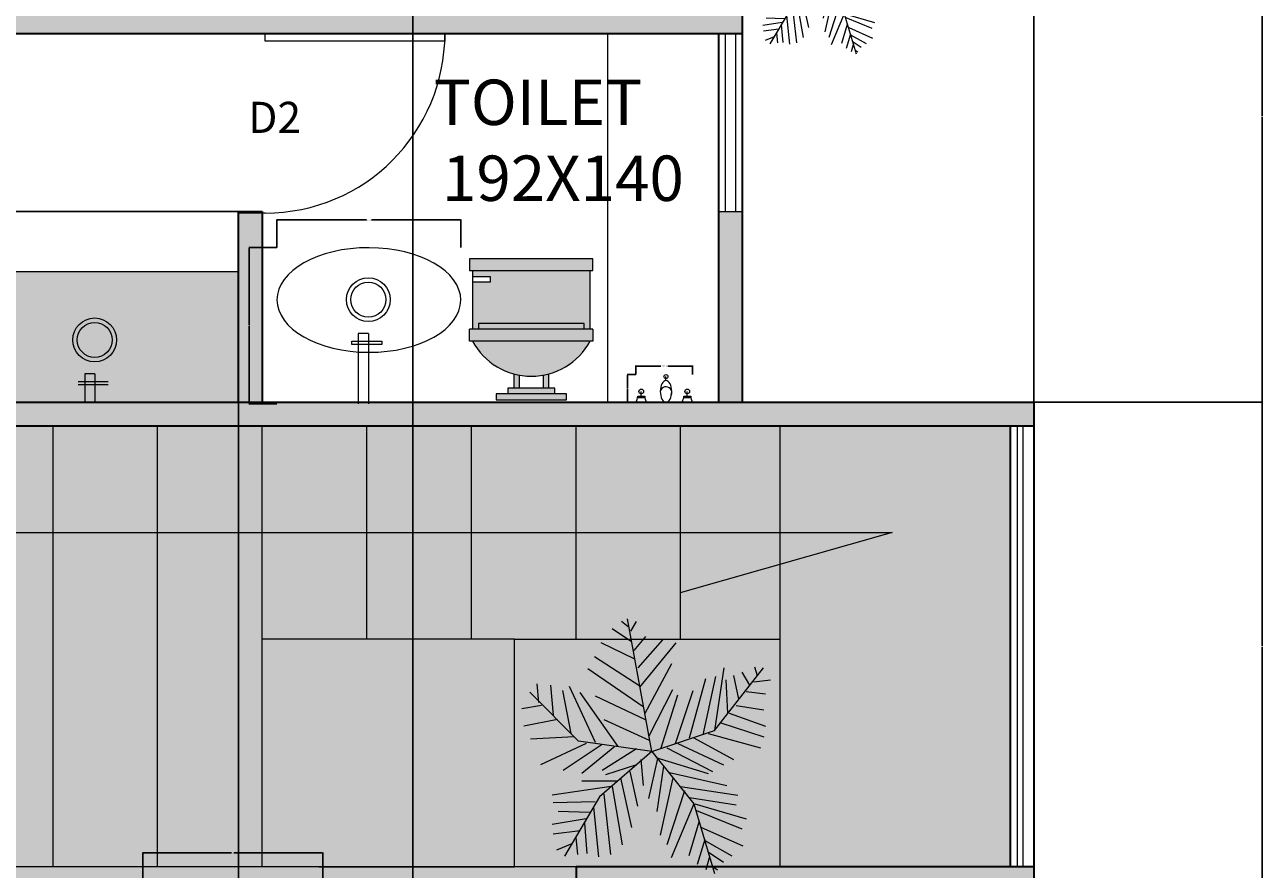
# Model space of a CAD drawing. Units: inches. Extents: x 192 to 1361, y -1362 to 367.
# Tile 13 of 23: x 891 to 1361, y -775 to -454. Entities that reach past the tile are written whole.
import ezdxf

# ---------------------------------------------------------------- set-up
doc = ezdxf.new("R2010")
doc.units = ezdxf.units.IN
doc.header["$MEASUREMENT"] = 0
for name, color, linetype, lineweight in [('A-ANNO-DIMS', 2, 'Continuous', 18), ('A-ANNO-SYMB', 7, 'Continuous', 18), ('A-AREA-IDEN', 7, 'Continuous', 18), ('A-DOOR', 4, 'Continuous', 18), ('A-FLOR-CASE', 32, 'Continuous', 18), ('A-FLOR-FIXT', 8, 'Continuous', 18), ('A-FLOR-STRS', 7, 'Continuous', 18), ('A-WALL-PATT', 250, 'Continuous', 13), ('lawn', 96, 'Continuous', 13), ('text', 7, 'Continuous', 18), ('walls', 7, 'Continuous', 35), ('windows', 4, 'Continuous', 18)]:
    doc.layers.add(name, color=color, linetype=linetype, lineweight=lineweight)
for name, color, linetype, lineweight, true_color in [('A-FLOR-CASE-PATT', 9, 'Continuous', 13, 0xc7c8ca), ('A-FLOR-FIXT-PATT', 251, 'Continuous', 13, 0x636466), ('A-FLOR-STRS-PATT', 252, 'Continuous', 13, 0x939598)]:
    doc.layers.add(name, color=color, linetype=linetype, lineweight=lineweight, true_color=true_color)
doc.styles.get("Standard").update_dxf_attribs({"font": 'arial.ttf'})
doc.dimstyles.get("Standard").update_dxf_attribs({"dimtxt": 0.18, "dimasz": 0.18, "dimexe": 0.18, "dimexo": 0.0625, "dimgap": 0.09, "dimtad": 0, "dimtih": 1, "dimtoh": 1, "dimzin": 0, "dimdsep": 46, "dimlunit": 3, "dimtxsty": 'Standard', "dimcen": 0.09, "dimadec": 0, "dimazin": 0, "dimtfac": 1, "dimtofl": 0, "dimtmove": 0, "dimatfit": 3, "dimfxl": 1, "dimtolj": 1, "dimtzin": 0, "dimarcsym": 0})

# ---------------------------------------------------------------- blocks, each defined once
blk = doc.blocks.new('*U2')
for p, q in [((0, 0), (0, -6)), ((40, 0), (40, -6))]:
    blk.add_line(p, q)
blk.add_lwpolyline([(0, 0), (0, 40), (1.75, 40), (1.75, 0)], close=True)
blk.add_arc((0, 0), 40, 0, 90)
blk = doc.blocks.new('*U4')
for p, q in [((-10.186, 53.64), (-13.084, 55.962)), ((0, 0), (-10.5, 57)), ((-9.099, 51.782), (-6.563, 55.962)), ((-8.737, 47.138), (-17.069, 52.711)), ((-7.65, 43.423), (-2.578, 49.46)), ((-5.839, 35.992), (4.667, 48.067)), ((-7.288, 39.707), (-21.778, 46.673)), ((-5.114, 27.632), (10.463, 46.673)), ((-5.114, 28.097), (-24.676, 40.636)), ((-2.941, 16.486), (8.652, 37.85)), ((-3.665, 19.273), (-27.574, 35.527)), ((22.055, 7.198), (27.489, 32.277)), ((27, 9), (48, 36)), ((27.127, 9.056), (31.112, 35.992)), ((35.096, 32.741), (37.27, 22.524)), ((38.719, 34.134), (41.979, 28.561)), ((44.153, 36.456), (45.239, 32.741)), ((-48.585, 21.131), (-49.309, 29.026)), ((-43.513, 28.561), (-42.427, 15.558)), ((-35.544, 28.097), (-24.314, 3.947)), ((-1.129, 6.734), (9.014, 26.704)), ((16.259, 5.805), (23.142, 31.348)), ((31.836, 30.883), (32.561, 16.486)), ((43.791, 29.954), (51.036, 30.883)), ((-31.5, 4.5), (-52.5, 25.5)), ((-38.442, 26.239), (-34.819, 7.663)), ((-14.533, 2.09), (-30.834, 25.31)), ((-24.314, 23.917), (-2.941, 13.7)), ((3.942, 1.625), (11.187, 24.381)), ((10.101, 3.483), (17.708, 26.239)), ((40.53, 25.775), (48.862, 24.846)), ((-47.498, 19.737), (-55.83, 18.344)), ((33.285, 16.486), (48.862, 10.913)), ((36.183, 19.737), (48.137, 17.88)), ((-40.615, 13.7), (-55.105, 10.913)), ((-20.691, 13.7), (-1.129, 4.876)), ((29.662, 12.307), (48.137, 6.269)), ((-33.37, 6.269), (-52.207, 5.34)), ((0, 0), (27, 9)), ((18.07, 5.805), (35.096, -3.483)), ((24.229, 7.663), (46.688, 1.625)), ((-28.299, 3.483), (-47.86, -5.805)), ((-21.416, 3.018), (-38.079, -8.128)), ((0, 0), (-31.5, 4.5)), ((-15.982, 2.09), (-30.11, -9.521)), ((0, 0), (-22.5, -19.5)), ((-6.563, 1.161), (-21.416, -8.128)), ((0, 0), (18, -22.5)), ((6.478, 1.625), (26.04, -8.592)), ((11.187, 3.483), (30.749, -5.805)), ((-4.752, -3.483), (-3.665, -14.629)), ((2.493, -3.019), (-1.491, -20.202)), ((1.769, -2.555), (24.229, -9.521)), ((-6.563, -5.805), (-19.967, -9.985)), ((-9.461, -8.592), (-6.201, -23.453)), ((5.029, -6.27), (2.131, -25.775)), ((7.565, -9.056), (32.198, -14.629)), ((-17.431, -15.094), (-42.789, -18.809)), ((-15.257, -12.772), (-30.11, -12.772)), ((-17.069, -15.094), (-12.721, -40.172)), ((-13.446, -11.378), (-8.737, -32.741)), ((9.014, -11.378), (3.58, -35.992)), ((12.274, -15.094), (36.907, -18.809)), ((-22.5, -19.5), (-37.5, -45)), ((-20.691, -18.345), (-17.793, -44.352)), ((14.085, -16.951), (6.478, -40.172)), ((16.259, -19.738), (36.183, -22.989)), ((-24.314, -21.596), (-42.427, -22.06)), ((-26.849, -26.24), (-40.253, -25.775)), ((-25.038, -23.918), (-22.865, -45.281)), ((18.07, -22.524), (8.289, -45.745)), ((18, -22.5), (27, -52.5)), ((18.433, -22.524), (40.53, -29.026)), ((19.157, -25.311), (38.719, -33.206)), ((-28.299, -29.026), (-42.789, -31.348)), ((-29.023, -30.884), (-27.936, -43.887)), ((20.244, -30.419), (15.897, -44.816)), ((-30.834, -34.135), (-42.427, -35.528)), ((-32.646, -36.921), (-31.921, -44.352)), ((21.331, -32.741), (39.081, -40.636)), ((-34.457, -39.708), (-40.978, -42.494)), ((22.78, -37.85), (19.519, -48.532)), ((22.78, -38.314), (34.372, -44.816)), ((24.591, -45.745), (23.142, -50.854)), ((24.591, -43.423), (30.749, -47.603)), ((26.764, -49.925), (28.213, -50.854))]:
    blk.add_line(p, q)
blk = doc.blocks.new('*U18')
for p, q in [((-10, 22), (-10, 12)), ((10, 12), (10, 22)), ((-10, 21), (-7, 21)), ((-7, 20), (-10, 20)), ((-7, 21), (-7, 20)), ((9, 13), (-9, 13)), ((-9, 13), (-9, 12)), ((9, 12), (9, 13)), ((10.5, 12), (-10.5, 12)), ((-10.5, 10), (-10.5, 12)), ((10.5, 12), (10.5, 10)), ((10.5, 10), (-10.5, 10)), ((-3, 4.4065), (-3, 2)), ((3, 2), (3, 4.4065)), ((-2, 2), (-2, 4.1658)), ((2, 4.1658), (2, 2)), ((4, 2), (-4, 2)), ((-4, 2), (-4, 1)), ((4, 1), (4, 2))]:
    blk.add_line(p, q)
for points in [[(10.5, 22), (10.5, 24), (-10.5, 24), (-10.5, 22)], [(6, 0), (6, 1), (-6, 1), (-6, 0)]]:
    blk.add_lwpolyline(points, close=True)
blk.add_arc((0, 15.3333), 11.3333, 208.0725, 331.9275)
blk = doc.blocks.new('BASIN-OVAL-WITH-TAP')
for p, q in [((-0.13, -12.72), (-4, -12.74)), ((-4, -12.74), (-4, -39.43)), ((-0.13, -12.72), (-0.13, -39.43)), ((-6.48, -15.66), (4.91, -15.61)), ((-6.47, -16.92), (-6.48, -15.66)), ((4.94, -16.86), (-6.47, -16.92))]:
    blk.add_line(p, q)
for radius in [8.31, 6.64]:
    blk.add_circle((-0.19, 0.14), radius)
at = {"extrusion": (0, 0, -1)}
blk.add_ellipse((0, 0), major_axis=(-34.9, 0.1), ratio=0.56899, dxfattribs=at)
blk = doc.blocks.new('BATH-MIXER-TWIN-HANDLE')
for p, q in [((0, 4.11), (0, 5.63)), ((-10.73, -2.32), (-8.02, -2.36)), ((-10.7, -1.84), (-8.05, -1.84)), ((-9.38, -1.84), (-9.38, -0.03)), ((6.73, -2.31), (9.44, -2.32)), ((6.76, -1.84), (9.41, -1.84)), ((8.08, -1.84), (8.08, -0.03))]:
    blk.add_line(p, q)
for centre, radius in [((0, 5.63), 0.761), ((-9.38, -0.03), 0.904), ((8.08, -0.03), 0.904)]:
    blk.add_circle(centre, radius)
for centre, radius, start, end in [((0, -0.5), 2.23, 336.3452, 166.942), ((-14.82, -1.84), 4.11, 326.5495, 0), ((-3.94, -1.84), 4.11, 180, 213.4505), ((2.65, -1.84), 4.11, 326.5495, 0), ((13.52, -1.84), 4.11, 180, 213.4505)]:
    blk.add_arc(centre, radius, start, end)
at = {"extrusion": (0, 0, -1)}
blk.add_ellipse((0, 0), major_axis=(0, -4.11), ratio=0.528671, dxfattribs=at)
blk = doc.blocks.new('*D33')
at = {"layer": 'A-ANNO-DIMS', "color": 0, "lineweight": -2, "transparency": 16777216}
for p, q in [((986.19, -538.74), (986.19, -528.14)), ((986.37, -528.32), (1020.18, -528.32)), ((1055.87, -528.32), (1022.06, -528.32)), ((1056.05, -538.74), (1056.05, -528.14))]:
    blk.add_line(p, q, dxfattribs=at)
at = {"layer": 'A-ANNO-DIMS', "color": 0, "transparency": 16777216}
for points in [[(986.37, -528.29), (986.37, -528.35), (986.19, -528.32)], [(1055.87, -528.29), (1055.87, -528.35), (1056.05, -528.32)]]:
    blk.add_solid(points, dxfattribs=at)
at = {"layer": 'Defpoints', "color": 0, "transparency": 16777216}
for p in [(1056.05, -528.32), (986.19, -538.8), (1056.05, -538.8)]:
    blk.add_point(p, dxfattribs=at)
at = {"layer": 'A-ANNO-DIMS', "color": 0, "transparency": 16777216, "insert": (1021.12, -528.32), "char_height": 0.18, "attachment_point": 5}
blk.add_mtext('\\A1;BASIN 70 TYP.', dxfattribs=at)
blk = doc.blocks.new('*D34')
at = {"layer": 'A-ANNO-DIMS', "color": 0, "lineweight": -2, "transparency": 16777216}
for p, q in [((986.13, -538.8), (975.54, -538.8)), ((975.72, -538.98), (975.72, -568.28)), ((975.72, -597.95), (975.72, -568.65)), ((986.13, -598.13), (975.54, -598.13))]:
    blk.add_line(p, q, dxfattribs=at)
at = {"layer": 'A-ANNO-DIMS', "color": 0, "transparency": 16777216}
for points in [[(975.69, -538.98), (975.75, -538.98), (975.72, -538.8)], [(975.69, -597.95), (975.75, -597.95), (975.72, -598.13)]]:
    blk.add_solid(points, dxfattribs=at)
at = {"layer": 'Defpoints', "color": 0, "transparency": 16777216}
for p in [(975.72, -538.8), (986.19, -538.8), (986.19, -598.13)]:
    blk.add_point(p, dxfattribs=at)
at = {"layer": 'A-ANNO-DIMS', "color": 0, "transparency": 16777216, "insert": (975.72, -568.47), "char_height": 0.18, "attachment_point": 5}
blk.add_mtext('\\A1;59 TYP.', dxfattribs=at)
blk = doc.blocks.new('*D35')
at = {"layer": 'A-ANNO-DIMS', "color": 0, "lineweight": -2, "transparency": 16777216}
for p, q in [((1122.52, -586.94), (1122.52, -583.6)), ((1122.7, -583.78), (1131.93, -583.78)), ((1143.81, -583.78), (1134.58, -583.78)), ((1143.99, -586.94), (1143.99, -583.6))]:
    blk.add_line(p, q, dxfattribs=at)
at = {"layer": 'A-ANNO-DIMS', "color": 0, "transparency": 16777216}
for points in [[(1122.7, -583.75), (1122.7, -583.81), (1122.52, -583.78)], [(1143.81, -583.75), (1143.81, -583.81), (1143.99, -583.78)]]:
    blk.add_solid(points, dxfattribs=at)
at = {"layer": 'Defpoints', "color": 0, "transparency": 16777216}
for p in [(1122.52, -587), (1143.99, -583.78), (1143.99, -587)]:
    blk.add_point(p, dxfattribs=at)
at = {"layer": 'A-ANNO-DIMS', "color": 0, "transparency": 16777216, "insert": (1133.26, -583.78), "char_height": 0.18, "attachment_point": 5}
blk.add_mtext('\\A1;BATH MIXER 21 TYP.', dxfattribs=at)
blk = doc.blocks.new('*D36')
at = {"layer": 'A-ANNO-DIMS', "color": 0, "lineweight": -2, "transparency": 16777216}
for p, q in [((1122.46, -587), (1119.12, -587)), ((1119.3, -587.18), (1119.3, -592.07)), ((1119.3, -597.32), (1119.3, -592.43)), ((1122.46, -597.5), (1119.12, -597.5))]:
    blk.add_line(p, q, dxfattribs=at)
at = {"layer": 'A-ANNO-DIMS', "color": 0, "transparency": 16777216}
for points in [[(1119.27, -587.18), (1119.33, -587.18), (1119.3, -587)], [(1119.27, -597.32), (1119.33, -597.32), (1119.3, -597.5)]]:
    blk.add_solid(points, dxfattribs=at)
at = {"layer": 'Defpoints', "color": 0, "transparency": 16777216}
for p in [(1119.3, -587), (1122.52, -587), (1122.52, -597.5)]:
    blk.add_point(p, dxfattribs=at)
at = {"layer": 'A-ANNO-DIMS', "color": 0, "transparency": 16777216, "insert": (1119.3, -592.25), "char_height": 0.18, "attachment_point": 5}
blk.add_mtext('\\A1;10 TYP.', dxfattribs=at)
blk = doc.blocks.new('*D41')
at = {"layer": 'A-ANNO-DIMS', "color": 0, "lineweight": -2, "transparency": 16777216}
for p, q in [((935.27, -778.85), (935.27, -768.47)), ((935.45, -768.65), (969.03, -768.65)), ((1003.45, -768.65), (969.87, -768.65)), ((1003.63, -778.85), (1003.63, -768.47))]:
    blk.add_line(p, q, dxfattribs=at)
at = {"layer": 'A-ANNO-DIMS', "color": 0, "transparency": 16777216}
for points in [[(935.45, -768.62), (935.45, -768.68), (935.27, -768.65)], [(1003.45, -768.62), (1003.45, -768.68), (1003.63, -768.65)]]:
    blk.add_solid(points, dxfattribs=at)
at = {"layer": 'Defpoints', "color": 0, "transparency": 16777216}
for p in [(935.27, -768.65), (935.27, -778.91), (1003.63, -778.91)]:
    blk.add_point(p, dxfattribs=at)
at = {"layer": 'A-ANNO-DIMS', "color": 0, "transparency": 16777216, "insert": (969.45, -768.65), "char_height": 0.18, "attachment_point": 5}
blk.add_mtext('\\A1;TV 68', dxfattribs=at)
blk = doc.blocks.new('*D52')
at = {"layer": 'A-ANNO-DIMS', "color": 0, "lineweight": -2, "transparency": 16777216}
for p, q in [((1162.8, -60.44), (1162.8, 367.39)), ((1162.98, 367.21), (1217.73, 367.21)), ((1273.39, 367.21), (1218.64, 367.21)), ((1273.57, -597.44), (1273.57, 367.39))]:
    blk.add_line(p, q, dxfattribs=at)
at = {"layer": 'A-ANNO-DIMS', "color": 0, "transparency": 16777216}
for points in [[(1162.98, 367.24), (1162.98, 367.18), (1162.8, 367.21)], [(1273.39, 367.24), (1273.39, 367.18), (1273.57, 367.21)]]:
    blk.add_solid(points, dxfattribs=at)
at = {"layer": 'Defpoints', "color": 0, "transparency": 16777216}
for p in [(1273.57, 367.21), (1162.8, -60.5), (1273.57, -597.5)]:
    blk.add_point(p, dxfattribs=at)
at = {"layer": 'A-ANNO-DIMS', "color": 0, "transparency": 16777216, "insert": (1218.18, 367.21), "char_height": 0.18, "attachment_point": 5}
blk.add_mtext('\\A1;110.76', dxfattribs=at)
blk = doc.blocks.new('*D57')
at = {"layer": 'A-ANNO-DIMS', "color": 0, "lineweight": -2, "transparency": 16777216}
for p, q in [((1162.87, -380.68), (1360.41, -380.68)), ((1360.23, -380.86), (1360.23, -488.91)), ((1360.23, -597.32), (1360.23, -489.27)), ((1162.87, -597.5), (1360.41, -597.5))]:
    blk.add_line(p, q, dxfattribs=at)
at = {"layer": 'A-ANNO-DIMS', "color": 0, "transparency": 16777216}
for points in [[(1360.2, -380.86), (1360.26, -380.86), (1360.23, -380.68)], [(1360.2, -597.32), (1360.26, -597.32), (1360.23, -597.5)]]:
    blk.add_solid(points, dxfattribs=at)
at = {"layer": 'Defpoints', "color": 0, "transparency": 16777216}
for p in [(1162.8, -380.68), (1162.8, -597.5), (1360.23, -597.5)]:
    blk.add_point(p, dxfattribs=at)
at = {"layer": 'A-ANNO-DIMS', "color": 0, "transparency": 16777216, "insert": (1360.23, -489.09), "char_height": 0.18, "attachment_point": 5}
blk.add_mtext('\\A1;216.82', dxfattribs=at)
blk = doc.blocks.new('*D58')
at = {"layer": 'A-ANNO-DIMS', "color": 0, "lineweight": -2, "transparency": 16777216}
for p, q in [((1273.63, -597.5), (1360.41, -597.5)), ((1360.23, -597.68), (1360.23, -690.01)), ((1360.23, -782.71), (1360.23, -690.38)), ((1273.63, -782.89), (1360.41, -782.89))]:
    blk.add_line(p, q, dxfattribs=at)
at = {"layer": 'A-ANNO-DIMS', "color": 0, "transparency": 16777216}
for points in [[(1360.2, -597.68), (1360.26, -597.68), (1360.23, -597.5)], [(1360.2, -782.71), (1360.26, -782.71), (1360.23, -782.89)]]:
    blk.add_solid(points, dxfattribs=at)
at = {"layer": 'Defpoints', "color": 0, "transparency": 16777216}
for p in [(1273.57, -597.5), (1273.57, -782.89), (1360.23, -782.89)]:
    blk.add_point(p, dxfattribs=at)
at = {"layer": 'A-ANNO-DIMS', "color": 0, "transparency": 16777216, "insert": (1360.23, -690.2), "char_height": 0.18, "attachment_point": 5}
blk.add_mtext('\\A1;185.4', dxfattribs=at)
blk = doc.blocks.new('*D68')
at = {"layer": 'A-ANNO-DIMS', "color": 0, "lineweight": -2, "transparency": 16777216}
for p, q in [((856.57, -597.56), (856.57, -1200.05)), ((971.58, -597.56), (971.58, -1200.05)), ((856.75, -1199.87), (913.79, -1199.87)), ((971.4, -1199.87), (914.36, -1199.87))]:
    blk.add_line(p, q, dxfattribs=at)
at = {"layer": 'A-ANNO-DIMS', "color": 0, "transparency": 16777216}
for points in [[(856.75, -1199.84), (856.75, -1199.9), (856.57, -1199.87)], [(971.4, -1199.84), (971.4, -1199.9), (971.58, -1199.87)]]:
    blk.add_solid(points, dxfattribs=at)
at = {"layer": 'Defpoints', "color": 0, "transparency": 16777216}
for p in [(856.57, -597.5), (971.58, -597.5), (971.58, -1199.87)]:
    blk.add_point(p, dxfattribs=at)
at = {"layer": 'A-ANNO-DIMS', "color": 0, "transparency": 16777216, "insert": (914.07, -1199.87), "char_height": 0.18, "attachment_point": 5}
blk.add_mtext('\\A1;115', dxfattribs=at)
blk = doc.blocks.new('*D69')
at = {"layer": 'A-ANNO-DIMS', "color": 0, "lineweight": -2, "transparency": 16777216}
for p, q in [((981.75, -457.5), (192.16, -457.5)), ((192.34, -457.68), (192.34, -491.13)), ((192.34, -524.95), (192.34, -491.5)), ((980.52, -525.13), (192.16, -525.13))]:
    blk.add_line(p, q, dxfattribs=at)
at = {"layer": 'A-ANNO-DIMS', "color": 0, "transparency": 16777216}
for points in [[(192.31, -457.68), (192.37, -457.68), (192.34, -457.5)], [(192.31, -524.95), (192.37, -524.95), (192.34, -525.13)]]:
    blk.add_solid(points, dxfattribs=at)
at = {"layer": 'Defpoints', "color": 0, "transparency": 16777216}
for p in [(981.81, -457.5), (192.34, -525.13), (980.58, -525.13)]:
    blk.add_point(p, dxfattribs=at)
at = {"layer": 'A-ANNO-DIMS', "color": 0, "transparency": 16777216, "insert": (192.34, -491.31), "char_height": 0.18, "attachment_point": 5}
blk.add_mtext('\\A1;67.63', dxfattribs=at)
blk = doc.blocks.new('*D72')
at = {"layer": 'A-ANNO-DIMS', "color": 0, "lineweight": -2, "transparency": 16777216}
for p, q in [((835.08, -1067.56), (835.08, 367.39)), ((835.26, 367.21), (935.95, 367.21)), ((1037.58, 367.21), (936.88, 367.21)), ((1037.76, -1067.56), (1037.76, 367.39))]:
    blk.add_line(p, q, dxfattribs=at)
at = {"layer": 'A-ANNO-DIMS', "color": 0, "transparency": 16777216}
for points in [[(835.26, 367.24), (835.26, 367.18), (835.08, 367.21)], [(1037.58, 367.24), (1037.58, 367.18), (1037.76, 367.21)]]:
    blk.add_solid(points, dxfattribs=at)
at = {"layer": 'Defpoints', "color": 0, "transparency": 16777216}
for p in [(1037.76, 367.21), (835.08, -1067.62), (1037.76, -1067.62)]:
    blk.add_point(p, dxfattribs=at)
at = {"layer": 'A-ANNO-DIMS', "color": 0, "transparency": 16777216, "insert": (936.42, 367.21), "char_height": 0.18, "attachment_point": 5}
blk.add_mtext('\\A1;202.68', dxfattribs=at)

msp = doc.modelspace()

# ---------------------------------------------------------------- hatches: boundary and pattern name
at = {"layer": 'A-FLOR-CASE-PATT'}
h = msp.add_hatch(color=256, dxfattribs=at)
h.dxf.hatch_style = 1
h.paths.add_polyline_path([(971.5799, -548.0101), (856.5691, -548.0101), (856.5691, -597.4996), (971.5799, -597.4996)])
h = msp.add_hatch(color=256, dxfattribs=at)
h.dxf.hatch_style = 1
h.paths.add_polyline_path([(1099.8366, -773.892), (784.8041, -773.892), (784.8041, -797.1415), (1099.8366, -797.1415)])
at = {"layer": 'A-FLOR-FIXT-PATT'}
h = msp.add_hatch(color=256, dxfattribs=at)
h.dxf.hatch_style = 1
h.paths.add_polyline_path([(1106.1981, -543.0682), (1059.375, -543.0682), (1059.375, -547.5275), (1106.1981, -547.5275)])
h.paths.add_polyline_path([(1105.0833, -547.5275), (1060.4898, -547.5275), (1060.4898, -549.7572), (1067.1788, -549.7572), (1067.1788, -551.9869), (1060.4898, -551.9869), (1060.4898, -569.8243), (1062.7195, -569.8243), (1062.7195, -567.5946), (1102.8536, -567.5946), (1102.8536, -569.8243), (1105.0833, -569.8243)])
h.paths.add_polyline_path([(1102.8536, -567.5946), (1062.7195, -567.5946), (1062.7195, -569.8243), (1102.8536, -569.8243)], flags=17)
h.paths.add_polyline_path([(1106.1981, -569.8243), (1059.375, -569.8243), (1059.375, -574.2836), (1106.1981, -574.2836)])
h.paths.add_polyline_path([(1105.0833, -574.2836), (1060.4898, -574.2836, 0.60000216)])
h.paths.add_polyline_path([(1078.3272, -587.2651, -0.0226287), (1076.0975, -586.7603), (1076.0975, -592.121), (1078.3272, -592.121)])
h.paths.add_polyline_path([(1089.4756, -586.7603, -0.0226287), (1087.2459, -587.2651), (1087.2459, -592.121), (1089.4756, -592.121)])
h.paths.add_polyline_path([(1091.7053, -592.121), (1073.8679, -592.121), (1073.8679, -594.3507), (1091.7053, -594.3507)])
h.paths.add_polyline_path([(1096.1646, -594.3507), (1069.4085, -594.3507), (1069.4085, -596.5804), (1096.1646, -596.5804)])
at = {"layer": 'A-FLOR-STRS-PATT'}
h = msp.add_hatch(color=256, dxfattribs=at)
h.dxf.hatch_style = 1
h.paths.add_polyline_path([(821.7257, -606.4996), (784.8041, -606.4996), (784.8041, -773.892), (821.7257, -773.892)])
h.paths.add_polyline_path([(861.4265, -606.4996), (821.7257, -606.4996), (821.7257, -773.892), (861.4265, -773.892)])
h.paths.add_polyline_path([(940.828, -606.4996), (901.1272, -606.4996), (901.1272, -773.892), (940.828, -773.892)])
h.paths.add_polyline_path([(901.1272, -606.4996), (861.4265, -606.4996), (861.4265, -773.892), (901.1272, -773.892)])
h.paths.add_polyline_path([(980.5288, -687.5154), (980.5288, -606.4996), (940.828, -606.4996), (940.828, -773.892), (980.5288, -773.892)])
h.paths.add_polyline_path([(1020.2295, -606.4996), (980.5288, -606.4996), (980.5288, -687.5154), (1020.2295, -687.5154)])
h.paths.add_polyline_path([(1059.9303, -606.4996), (1020.2295, -606.4996), (1020.2295, -687.5154), (1059.9303, -687.5154)])
h.paths.add_polyline_path([(1099.631, -606.4996), (1059.9303, -606.4996), (1059.9303, -687.5154), (1076.4416, -687.5154), (1099.631, -687.5154)])
h.paths.add_polyline_path([(1139.3318, -606.4996), (1099.631, -606.4996), (1099.631, -687.5154), (1139.3318, -687.5154)])
h.paths.add_polyline_path([(1177.0582, -606.4996), (1139.3318, -606.4996), (1139.3318, -687.5154), (1177.0582, -687.5154)])
h.paths.add_polyline_path([(1264.5658, -606.4996), (1177.0582, -606.4996), (1177.0582, -687.5154), (1177.0582, -773.892), (1264.5658, -773.892)])
h = msp.add_hatch(color=256, dxfattribs=at)
h.dxf.hatch_style = 1
h.paths.add_polyline_path([(1076.4416, -687.5154), (980.5288, -687.5154), (980.5288, -773.892), (1076.4398, -773.892), (1076.4416, -762.6299)])
h = msp.add_hatch(color=256, dxfattribs=at)
h.dxf.hatch_style = 1
h.paths.add_polyline_path([(1177.0582, -687.5154), (1076.4416, -687.5154), (1076.4416, -762.6299), (1076.4398, -773.892), (1174.9036, -773.892), (1177.0582, -773.892)])
at = {"layer": 'A-WALL-PATT'}
h = msp.add_hatch(color=256, dxfattribs=at)
h.dxf.hatch_style = 1
h.paths.add_polyline_path([(309.5452, 191.102), (300.5452, 191.102), (300.5452, -126.898), (309.5452, -126.898), (309.5452, -117.898)])
h.paths.add_polyline_path([(420.798, 191.102), (337.3229, 191.102), (337.3229, 182.102), (420.798, 182.102)])
h.paths.add_polyline_path([(518.5452, 182.102), (625.4022, 182.102), (625.4022, 191.102), (509.5452, 191.102), (509.5452, 114.3262), (518.5452, 114.3262)])
h.paths.add_polyline_path([(842.5452, 191.102), (763.4438, 191.102), (763.4438, 182.102), (833.5452, 182.102), (833.5452, 161.1615), (836.8088, 161.1615), (842.5452, 161.1615)])
h.paths.add_polyline_path([(842.5452, -16.5675), (833.5452, -16.5675), (833.5452, -60.4996), (784.8041, -60.4996), (784.8041, -354.6796), (793.8041, -354.6796), (793.8041, -69.4996), (1094.1252, -69.4996), (1094.1252, -60.4996), (842.5452, -60.4996)])
h.paths.add_polyline_path([(518.5452, 36.602), (509.5452, 36.602), (509.5452, -117.898), (420.2204, -117.898), (420.2204, -126.898), (518.5452, -126.898)])
h.paths.add_polyline_path([(474.8041, -377.0384), (465.8041, -377.0384), (465.8041, -381.5384), (465.8041, -450.898), (537.5717, -450.898), (537.5717, -441.898), (474.8041, -441.898)])
h.paths.add_polyline_path([(1162.8041, -380.6763), (1204.3001, -380.6763), (1204.3001, -375.6763), (1195.1471, -375.6763), (1153.8041, -375.6763), (1153.8041, -448.4996), (856.5691, -448.4996), (856.5691, -457.4996), (1162.8041, -457.4996)])
h.paths.add_polyline_path([(1162.8041, -525.128), (1153.8041, -525.128), (1153.8041, -597.4996), (1162.8041, -597.4996)], flags=17)
h.paths.add_polyline_path([(1162.8041, -60.4996), (1153.8041, -60.4996), (1153.8041, -69.4996), (1153.8041, -177.4733), (1205.8889, -177.4733), (1205.8889, -172.4733), (1162.8041, -172.4733)])
h.paths.add_polyline_path([(980.5799, -525.686), (971.5799, -525.686), (971.5799, -597.4996), (980.5799, -597.4996)], flags=17)
h.paths.add_polyline_path([(856.5691, -448.4996), (798.7542, -448.4996), (784.8041, -448.4996), (784.8041, -457.4996), (847.5691, -457.4996), (847.5691, -597.4996), (784.8041, -597.4996), (784.8041, -606.4996), (1273.5658, -606.4996), (1273.5658, -597.4996), (856.5691, -597.4996)])
h.paths.add_polyline_path([(1273.5658, -773.892), (1099.8366, -773.892), (1099.8366, -851.9362), (1108.8366, -851.9362), (1108.8366, -782.892), (1273.5658, -782.892)])
h.paths.add_polyline_path([(1108.8366, -982.9214), (1099.8366, -982.9214), (1099.8366, -1067.6246), (1037.7563, -1067.6246), (1037.7563, -1076.6246), (1108.8366, -1076.6246)])
h.paths.add_polyline_path([(835.078, -1067.6246), (758.8458, -1067.6246), (758.8458, -940.2324), (749.8458, -940.2324), (749.8458, -963.172), (749.8458, -970.4644), (749.8458, -1076.6246), (835.078, -1076.6246)])
h.paths.add_polyline_path([(450.307, -1066.9838), (441.307, -1066.9838), (441.307, -1076.6246), (450.307, -1076.6246)])
h.paths.add_polyline_path([(492.8925, -756.4415), (274.8925, -756.4415), (274.8925, -765.4415), (492.8925, -765.4415)])
h.paths.add_polyline_path([(283.8925, -835.2244), (274.8925, -835.2244), (274.8925, -914.4415), (492.8925, -914.4415), (492.8925, -839.9415), (483.8925, -839.9415), (483.8925, -905.4415), (283.8925, -905.4415)])
h.paths.add_polyline_path([(283.8925, -441.898), (283.8925, -375.4296), (281.6021, -375.4296), (281.6021, -399.4121), (274.8925, -399.4121), (274.8925, -441.898), (274.8925, -684.5089), (283.8925, -684.5089)])

# ---------------------------------------------------------------- linework, layer by layer
at = {"layer": 'A-ANNO-SYMB'}
for p, q in [((755.4527, -647.0075), (1219.7014, -647.0075)), ((1219.7014, -647.0075), (1139.3318, -669.8647))]:
    msp.add_line(p, q, dxfattribs=at)
at = {"layer": 'A-FLOR-CASE'}
for p, q in [((971.5799, -548.0101), (856.5691, -548.0101)), ((1099.8366, -773.892), (784.8041, -773.892))]:
    msp.add_line(p, q, dxfattribs=at)
at = {"layer": 'A-FLOR-FIXT'}
for p, q in [((1111.7696, -597.4996), (1111.7696, -457.4996)), ((1026.0303, -574.3161), (1026.0303, -575.5711)), ((917.1324, -586.7091), (913.2627, -586.7276)), ((913.2627, -586.7276), (913.2627, -597.4996)), ((917.1324, -586.7091), (917.1324, -597.4996)), ((910.79, -589.6522), (922.1766, -589.5978)), ((922.2012, -590.8527), (910.796, -590.9072))]:
    msp.add_line(p, q, dxfattribs=at)
for radius in [8.3135, 6.638]:
    msp.add_circle((917.071, -573.8478), radius, dxfattribs=at)
at = {"layer": 'A-FLOR-STRS'}
for p, q in [((901.1272, -606.4996), (901.1272, -773.892)), ((901.1272, -606.4996), (901.1272, -773.892)), ((940.828, -606.4996), (940.828, -773.892)), ((940.828, -606.4996), (940.828, -773.892)), ((980.5288, -606.4996), (980.5288, -773.892)), ((980.5288, -606.4996), (980.5288, -773.892)), ((1020.2295, -606.4996), (1020.2295, -687.5154)), ((1020.2295, -606.4996), (1020.2295, -687.5154)), ((1059.9303, -606.4996), (1059.9303, -687.5154)), ((1059.9303, -606.4996), (1059.9303, -687.5154)), ((1099.631, -606.4996), (1099.631, -687.5154)), ((1099.631, -606.4996), (1099.631, -687.5154)), ((1139.3318, -606.4996), (1139.3318, -687.5154)), ((1139.3318, -606.4996), (1139.3318, -687.5154)), ((1177.0582, -606.4996), (1177.0582, -773.892)), ((1177.0582, -606.4996), (1177.0582, -773.892)), ((1076.4416, -687.5154), (980.5288, -687.5154)), ((980.5288, -687.5154), (980.5288, -773.892)), ((1076.4416, -687.5154), (980.5288, -687.5154)), ((1076.4416, -762.6299), (1076.4416, -687.5154)), ((1076.4416, -687.5154), (1177.0582, -687.5154)), ((1177.0582, -687.5154), (1177.0582, -773.892)), ((1076.4398, -773.892), (1076.4416, -762.6299)), ((1002.1255, -773.892), (1076.4398, -773.892)), ((1174.9036, -773.892), (1074.287, -773.892))]:
    msp.add_line(p, q, dxfattribs=at)
at = {"layer": 'walls'}
for p, q in [((1162.8041, -380.6763), (1162.8041, -457.4996)), ((856.5691, -457.4996), (1162.8041, -457.4996)), ((1153.8041, -457.4996), (1153.8041, -597.4996)), ((1162.8041, -457.4996), (1162.8041, -597.4996)), ((971.5799, -597.4996), (971.5799, -525.128)), ((971.5799, -525.128), (980.5799, -525.128)), ((980.5799, -525.128), (980.5799, -597.4996)), ((856.5691, -597.4996), (1273.5658, -597.4996)), ((1273.5658, -597.4996), (1273.5658, -782.892)), ((784.8041, -606.4996), (1273.5658, -606.4996)), ((1264.5658, -606.4996), (1264.5658, -773.892)), ((1099.8366, -773.892), (1099.8366, -1067.6246)), ((1273.5658, -773.892), (1099.8366, -773.892))]:
    msp.add_line(p, q, dxfattribs=at)
at = {"layer": 'windows'}
for p, q in [((1153.8041, -457.4996), (1162.8041, -457.4996)), ((1156.554, -525.128), (1156.554, -457.4996)), ((1160.4643, -525.128), (1160.4643, -457.4996)), ((1153.8041, -525.128), (1162.8041, -525.128)), ((1153.8041, -525.128), (1162.8041, -525.128)), ((1267.3719, -773.892), (1267.3719, -606.4996)), ((1269.3076, -606.4996), (1269.3076, -773.892)), ((1269.3076, -773.892), (1267.3719, -773.892))]:
    msp.add_line(p, q, dxfattribs=at)

# ---------------------------------------------------------------- block references
at = {"layer": 'A-DOOR', "xscale": 1.704660644661492, "yscale": 1.704660644661492, "zscale": 1.704660644661492, "rotation": 270}
msp.add_blockref('*U2', (981.8078, -457.4996), dxfattribs=at)
at = {"layer": 'A-FLOR-FIXT'}
for name, p in [('BASIN-OVAL-WITH-TAP', (1021.1195, -558.7063)), ('BATH-MIXER-TWIN-HANDLE', (1133.9025, -593.3925))]:
    msp.add_blockref(name, p, dxfattribs=at)
at = {"layer": 'A-FLOR-FIXT', "xscale": 2.229674534520691, "yscale": 2.229674534520691, "zscale": 2.229674534520691}
msp.add_blockref('*U18', (1082.7866, -596.5804), dxfattribs=at)
at = {"layer": 'lawn'}
for p, xscale, yscale, zscale in [((1192.4235, -438.5882), 0.5078671948952364, 0.5078671948952364, 0.5078671948952364), ((1128.537, -730.122), 0.8828807890770264, 0.8828807890770264, 0.8828807890770264)]:
    msp.add_blockref('*U4', p, dxfattribs=dict(at, xscale=xscale, yscale=yscale, zscale=zscale))

# ---------------------------------------------------------------- texts
at = {"layer": 'A-AREA-IDEN'}
for s, p in [('TOILET', (1045.7521, -492.2654)), ('192X140', (1048.8851, -521.0949))]:
    msp.add_text(s, height=17.23824, dxfattribs=at).set_placement(p)
at = {"layer": 'text'}
msp.add_text('D2', height=11.81288, dxfattribs=at).set_placement((975.3424, -495.264))

# ---------------------------------------------------------------- dimensions: what is measured, and where the dimension line sits
at = {"layer": 'A-ANNO-DIMS'}
for base, p1, p2, override, picture, middle in [((1037.7563, 367.2097), (835.078, -1067.6246), (1037.7563, -1067.6246), {"dimdec": 2, "dimlfac": 1, "dimrnd": 0, "dimzin": 0, "dimdsep": 46, "dimlunit": 2}, '*D72', (936.4171, 367.2097)), ((1273.5658, 367.2097), (1162.8041, -60.4996), (1273.5658, -597.4996), {"dimdec": 2, "dimlfac": 1, "dimrnd": 0, "dimzin": 0, "dimdsep": 46, "dimlunit": 2}, '*D52', (1218.185, 367.2097)), ((971.5799, -1199.8727), (856.5691, -597.4996), (971.5799, -597.4996), {"dimdec": 0, "dimlfac": 1, "dimrnd": 0, "dimzin": 0, "dimdsep": 46, "dimlunit": 2}, '*D68', (914.0745, -1199.8727))]:
    dim = msp.add_linear_dim(base=base, p1=p1, p2=p2, dimstyle='Standard', override=override, dxfattribs=at)
    dim.commit()
    dim.dimension.update_dxf_attribs({"geometry": picture, "text_midpoint": middle})
for base, p1, p2, override, picture, middle in [((1360.2331, -597.4996), (1162.8041, -380.6763), (1162.8041, -597.4996), {"dimdec": 2, "dimlfac": 1, "dimrnd": 0, "dimzin": 0, "dimdsep": 46, "dimlunit": 2}, '*D57', (1360.2331, -489.0879)), ((192.3425, -525.128), (981.8078, -457.4996), (980.5799, -525.128), {"dimdec": 2, "dimlfac": 1, "dimrnd": 0, "dimzin": 0, "dimdsep": 46, "dimlunit": 2}, '*D69', (192.3425, -491.3138)), ((1360.2331, -782.892), (1273.5658, -597.4996), (1273.5658, -782.892), {"dimdec": 1, "dimlfac": 1, "dimrnd": 0, "dimzin": 0, "dimdsep": 46, "dimlunit": 2}, '*D58', (1360.2331, -690.1958))]:
    dim = msp.add_linear_dim(base=base, p1=p1, p2=p2, angle=90, dimstyle='Standard', override=override, dxfattribs=at)
    dim.commit()
    dim.dimension.update_dxf_attribs({"geometry": picture, "text_midpoint": middle})
for base, p1, p2, text, picture, middle in [((1056.0459, -528.3197), (986.1932, -538.7976), (1056.0459, -538.7976), 'BASIN <> TYP.', '*D33', (1021.1195, -528.3197)), ((1143.9931, -583.7826), (1122.5178, -587.0039), (1143.9931, -587.0039), 'BATH MIXER <> TYP.', '*D35', (1133.2555, -583.7826))]:
    dim = msp.add_linear_dim(base=base, p1=p1, p2=p2, text=text, dimstyle='Standard', override={"dimdec": 0, "dimlfac": 1, "dimrnd": 0, "dimzin": 0, "dimdsep": 46, "dimlunit": 2}, dxfattribs=at)
    dim.commit()
    dim.dimension.update_dxf_attribs({"geometry": picture, "text_midpoint": middle})
for base, p1, p2, angle, text, picture, middle in [((975.7153, -538.7976), (986.1932, -598.1345), (986.1932, -538.7976), 90, '<> TYP.', '*D34', (975.7153, -568.4661)), ((1119.2965, -587.0039), (1122.5178, -597.4996), (1122.5178, -587.0039), 90, '<> TYP.', '*D36', (1119.2965, -592.2518)), ((935.2669, -768.6534), (1003.6315, -778.9081), (935.2669, -778.9081), 180, 'TV <>', '*D41', (969.4492, -768.6534))]:
    dim = msp.add_linear_dim(base=base, p1=p1, p2=p2, angle=angle, text=text, dimstyle='Standard', override={"dimdec": 0, "dimlfac": 1, "dimrnd": 0, "dimzin": 0, "dimdsep": 46, "dimlunit": 2}, dxfattribs=at)
    dim.commit()
    dim.dimension.update_dxf_attribs({"geometry": picture, "text_midpoint": middle})

doc.saveas('drawing.dxf')
